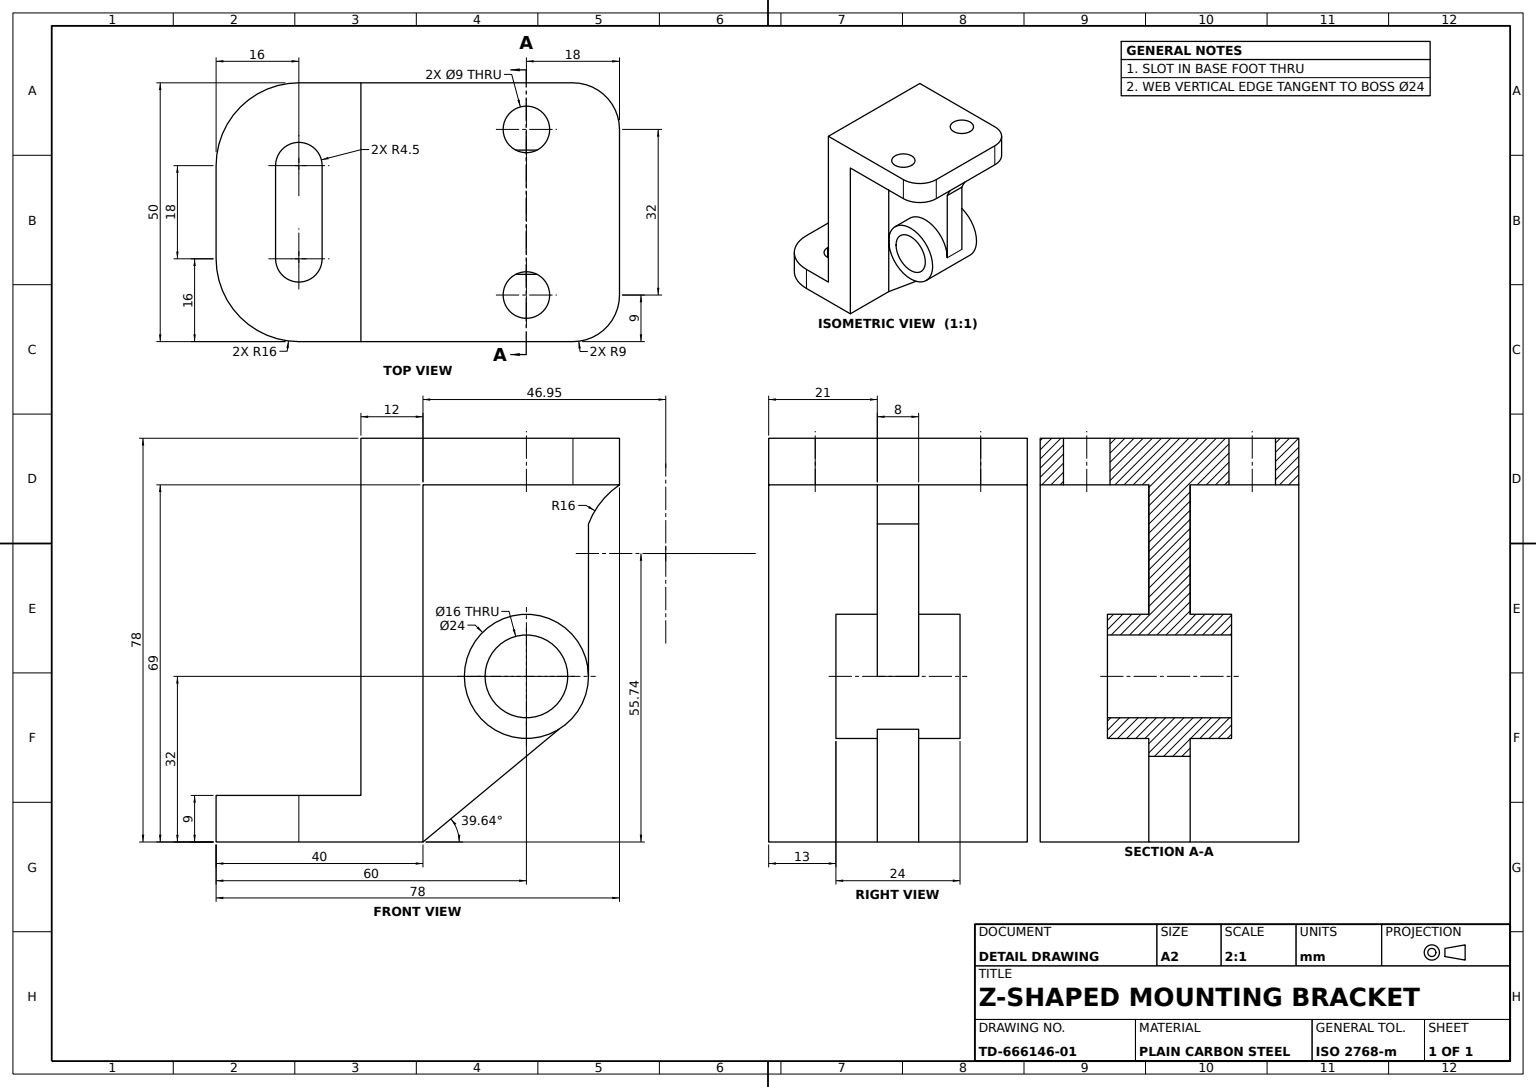
SolidWorks part; units mm, degrees
material "Plain Carbon Steel"
ref_plane "Front Plane" through (0, 0, 0) normal (0, 0, 1) x (1, 0, 0)
ref_plane "Top Plane" through (0, 0, 0) normal (0, 1, 0) x (1, 0, 0)
ref_plane "Right Plane" through (0, 0, 0) normal (1, 0, 0) x (0, 0, -1)
sketch "Base Foot Sketch" plane through (0, 0, 0) normal (0, 1, 0) x (1, 0, 0)
  line L0 (-9, 0.5) -> (9, 0.5)
  line L1 (-25, 20) -> (25, 20)
  line L2 (-25, 20) -> (-25, -4)
  line L3 (-9, -20) -> (9, -20)
  line L4 (25, 20) -> (25, -4)
  line L5 (-25, 20) -> (25, -20) construction
  line L6 (-25, -20) -> (25, 20) construction
  line L7 (-9, -8.5) -> (9, -8.5)
  arc A0 (9, -20) -> (25, -4) centre (9, -4) ccw
  arc A1 (-25, -4) -> (-9, -20) centre (-9, -4) ccw
  arc A2 (-9, 0.5) -> (-9, -8.5) centre (-9, -4) ccw
  arc A3 (9, -8.5) -> (9, 0.5) centre (9, -4) ccw
  point P0 (0, 0)
  dimension "D3" = 16
  dimension "D4" = 9
  dimension "D5" = 9
  dimension "D1" = 50
  dimension "D2" = 40
extrude "Base Foot with Slot" add sketch "Base Foot Sketch" along normal blind 9
sketch "Upright Wall Sketch" plane through (0, 0, -20) normal (0, 0, -1) x (-1, 0, 0)
  line L1 (-25, 9) -> (25, 9)
  line L2 (-25, 9) -> (-25, 78)
  line L3 (-25, 78) -> (25, 78)
  line L4 (25, 9) -> (25, 78)
  dimension "D1" = 50
  dimension "D2" = 69
extrude "Upright Wall" add sketch "Upright Wall Sketch" against normal blind 12
sketch "Top Flange Sketch" plane through (0, 78, 0) normal (0, 1, 0) x (1, 0, 0)
  line L0 (-25, 20) -> (-25, 49)
  line L1 (-16, 58) -> (16, 58)
  line L2 (25, 49) -> (25, 20)
  line L3 (-16, 58) -> (-16, 40)
  line L4 (-25, 20) -> (25, 20)
  arc A0 (16, 58) -> (25, 49) centre (16, 49) cw
  arc A1 (-25, 49) -> (-16, 58) centre (-16, 49) cw
  circle A2 centre (-16, 40) radius 4.5
  circle A3 centre (16, 40) radius 4.5
  point P8 (25, 58)
  point P11 (-25, 58)
  dimension "D3" = 9
  dimension "D5" = 9
  dimension "D6" = 9
  dimension "D1" = 50
  dimension "D2" = 38
  dimension "D4" = 18
extrude "Top Flange with 2 Holes" add sketch "Top Flange Sketch" against normal blind 9
sketch "Side Boss Sketch" plane through (0, 0, 0) normal (1, 0, 0) x (0, 0, -1)
  line L0 (20, 69) -> (20, 0) construction
  circle A0 centre (40, 32) radius 12
  circle A1 centre (40, 32) radius 8
  dimension "D1" = 24
  dimension "D2" = 16
  dimension "D3" = 32
  dimension "D4" = 20
extrude "Side Boss" add sketch "Side Boss Sketch" along normal mid plane 24 separate body
sketch "Boss Web Sketch" plane through (0, 0, 0) normal (1, 0, 0) x (0, 0, -1)
  line L0 (52, 32) -> (52, 61.4446)
  line L1 (20, 0) -> (46.2858, 21.778)
  line L2 (20, 0) -> (20, 69)
  line L3 (20, 69) -> (58, 69)
  circle A0 centre (40, 32) radius 12 construction
  arc A1 (52, 61.4446) -> (58, 69) centre (66.9466, 55.7351) cw
  arc A2 (52, 32) -> (46.2858, 21.778) centre (40, 32) cw
  dimension "D1" = 16
  dimension "D2" = 26.2858
  dimension "D3" = 46.9466
extrude "Boss Web" add sketch "Boss Web Sketch" along normal mid plane 8
sketch "Boss Bore Sketch" plane through (-4, 0, 0) normal (-1, 0, 0) x (0, 0, 1)
  circle A0 centre (-40, 32) radius 8
  dimension "D1" = 16
extrude "Boss Bore" cut sketch "Boss Bore Sketch" against normal through all
